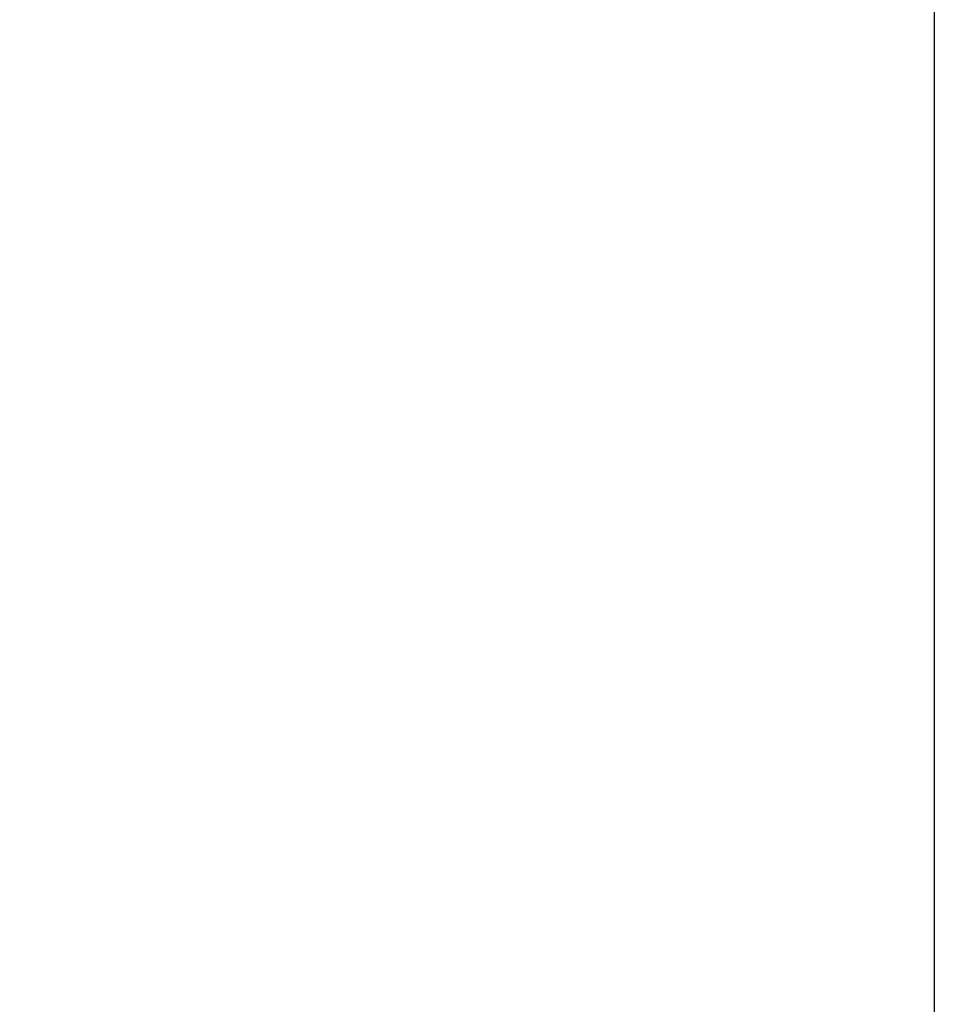
# Model space of a CAD drawing. Units: millimetres. Extents: x 595116 to 630915, y 909473 to 920225.
# Tile 92 of 134: x 629703 to 629744, y 919302 to 919346. Entities that reach past the tile are written whole.
import ezdxf

# ---------------------------------------------------------------- set-up
doc = ezdxf.new("R2010")
doc.units = ezdxf.units.MM
doc.layers.add('Dimension', color=3, linetype='Continuous', lineweight=18)
doc.styles.get("Standard").update_dxf_attribs({"font": 'arial.ttf'})
doc.dimstyles.new('ISO-25', dxfattribs={"dimtxt": 9, "dimasz": 6, "dimexe": 1.25, "dimexo": 0.625, "dimtad": 1, "dimlunit": 4, "dimtxsty": 'Standard', "dimcen": 2.5, "dimadec": 0, "dimazin": 0, "dimtfac": 1, "dimtmove": 0, "dimatfit": 3, "dimfxl": 1, "dimarcsym": 0})

# ---------------------------------------------------------------- blocks, each defined once
blk = doc.blocks.new('*D216')
at = {"layer": 'Defpoints', "color": 0, "transparency": 16777216}
for p in [(629505.041, 919411.828), (629743.541, 919411.928), (629743.541, 918832.378)]:
    blk.add_point(p, dxfattribs=at)
at = {"layer": 'Dimension', "color": 0, "lineweight": -2, "transparency": 16777216}
for p, q in [((629505.041, 919411.203), (629505.041, 918831.128)), ((629743.541, 919411.303), (629743.541, 918831.128)), ((629511.041, 918832.378), (629737.541, 918832.378))]:
    blk.add_line(p, q, dxfattribs=at)
at = {"layer": 'Dimension', "color": 0, "transparency": 16777216}
for points in [[(629511.041, 918833.378), (629511.041, 918831.378), (629505.041, 918832.378)], [(629737.541, 918833.378), (629737.541, 918831.378), (629743.541, 918832.378)]]:
    blk.add_solid(points, dxfattribs=at)
at = {"layer": 'Dimension', "color": 0, "transparency": 16777216, "insert": (629624.291, 918837.656), "char_height": 9, "attachment_point": 5}
blk.add_mtext('19\'-10 1/2"', dxfattribs=at)
blk = doc.blocks.new('*D220')
at = {"layer": 'Defpoints', "color": 0, "transparency": 16777216}
for p in [(629824.951, 920160.756), (629511.274, 919302.009), (629824.951, 919302.009)]:
    blk.add_point(p, dxfattribs=at)
at = {"layer": 'Dimension', "color": 0, "lineweight": -2, "transparency": 16777216}
for p, q in [((629511.274, 919302.634), (629511.274, 920162.006)), ((629824.951, 919302.634), (629824.951, 920162.006)), ((629517.274, 920160.756), (629818.951, 920160.756))]:
    blk.add_line(p, q, dxfattribs=at)
at = {"layer": 'Dimension', "color": 0, "transparency": 16777216}
for points in [[(629517.274, 920161.756), (629517.274, 920159.756), (629511.274, 920160.756)], [(629818.951, 920161.756), (629818.951, 920159.756), (629824.951, 920160.756)]]:
    blk.add_solid(points, dxfattribs=at)
at = {"layer": 'Dimension', "color": 0, "transparency": 16777216, "insert": (629668.113, 920166.035), "char_height": 9, "attachment_point": 5}
blk.add_mtext('26\'-1 1/2"', dxfattribs=at)

msp = doc.modelspace()

# ---------------------------------------------------------------- dimensions: what is measured, and where the dimension line sits
at = {"layer": 'Dimension'}
for base, p1, p2, picture, middle in [((629824.951, 920160.756), (629511.274, 919302.009), (629824.951, 919302.009), '*D220', (629668.113, 920166.035)), ((629743.541, 918832.378), (629505.041, 919411.828), (629743.541, 919411.928), '*D216', (629624.291, 918837.656))]:
    dim = msp.add_linear_dim(base=base, p1=p1, p2=p2, dimstyle='ISO-25', override={"dimdec": 1, "dimlfac": 1, "dimrnd": 0, "dimzin": 1, "dimdsep": 46, "dimlunit": 4, "dimfrac": 2}, dxfattribs=at)
    dim.commit()
    dim.dimension.update_dxf_attribs({"geometry": picture, "text_midpoint": middle})

doc.saveas('drawing.dxf')
